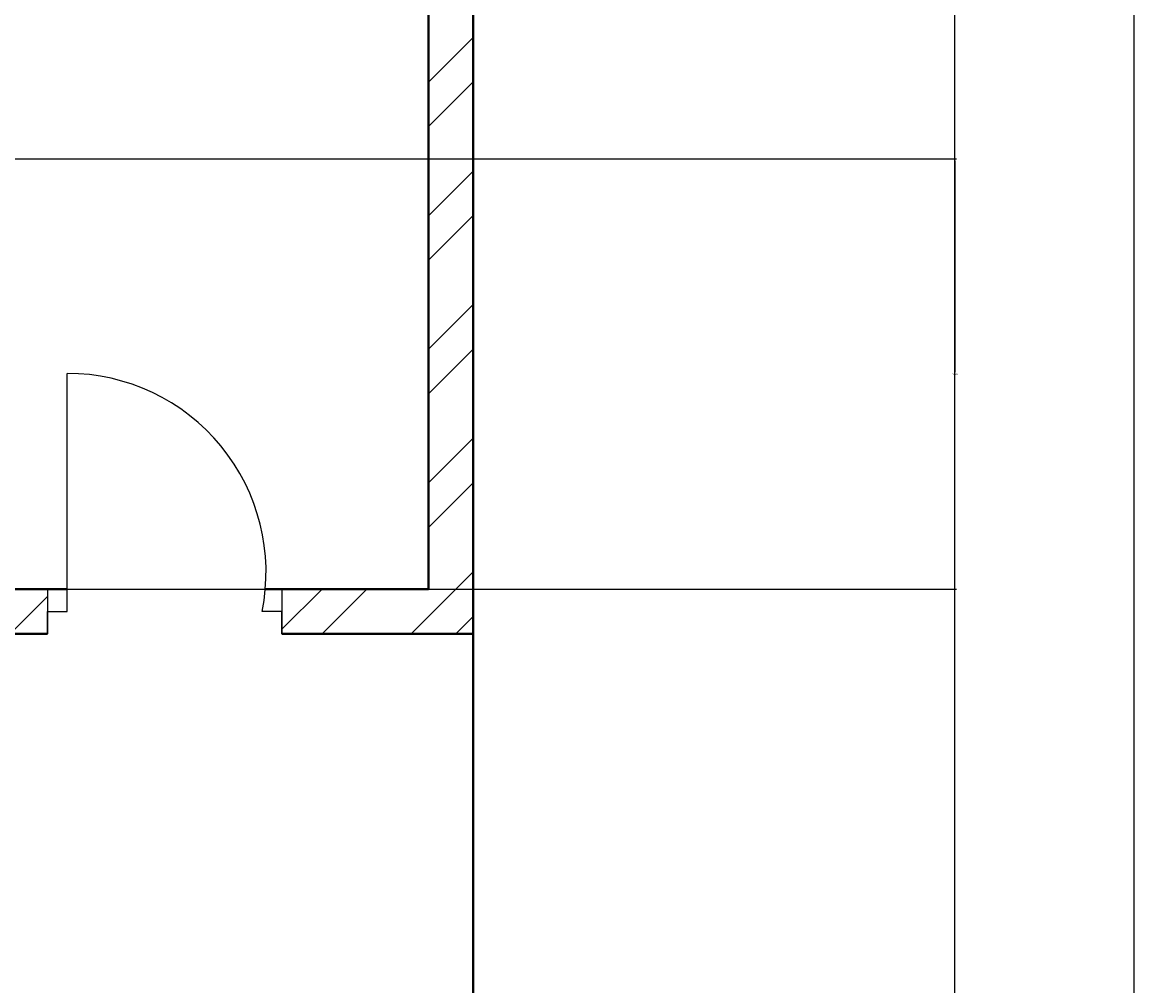
# Model space of a CAD drawing. Units: inches. Extents: x 1601 to 2297, y 1496 to 2631.
# Tile 30 of 57: x 2185 to 2297, y 1946 to 2043. Entities that reach past the tile are written whole.
import ezdxf

# ---------------------------------------------------------------- set-up
doc = ezdxf.new("R2010")
doc.units = ezdxf.units.IN
for name, color, linetype, lineweight in [('A-ANNO-DIMS', 2, 'Continuous', 18), ('A-ANNO-TTLB', 7, 'Continuous', 25), ('A-DOOR', 21, 'Continuous', 25), ('A-WALL', 7, 'Continuous', 40), ('A-WALL-PATT', 215, 'Continuous', 13)]:
    doc.layers.add(name, color=color, linetype=linetype, lineweight=lineweight)
doc.styles.get("Standard").update_dxf_attribs({"font": 'arial.ttf'})
doc.dimstyles.get("Standard").update_dxf_attribs({"dimtxt": 0.18, "dimasz": 0.18, "dimexe": 0.18, "dimexo": 0.0625, "dimgap": 0.09, "dimtad": 0, "dimtih": 1, "dimtoh": 1, "dimdec": 4, "dimzin": 0, "dimdsep": 46, "dimtxsty": 'Standard', "dimcen": 0.09, "dimadec": 0, "dimazin": 0, "dimtfac": 1, "dimtdec": 4, "dimtofl": 0, "dimtmove": 0, "dimatfit": 3, "dimfxl": 1, "dimtolj": 1, "dimtzin": 0, "dimarcsym": 0})

# ---------------------------------------------------------------- blocks, each defined once
blk = doc.blocks.new('*D29')
at = {"layer": 'A-ANNO-DIMS', "color": 0, "lineweight": -2, "transparency": 16777216}
for p, q in [((2230.6, 2532.33), (2279.27, 2532.33)), ((2279.09, 2532.15), (2279.09, 2084.01)), ((2279.09, 1635.51), (2279.09, 2083.64)), ((2230.6, 1635.33), (2279.27, 1635.33))]:
    blk.add_line(p, q, dxfattribs=at)
at = {"layer": 'A-ANNO-DIMS', "color": 0, "transparency": 16777216}
for points in [[(2279.06, 2532.15), (2279.12, 2532.15), (2279.09, 2532.33)], [(2279.06, 1635.51), (2279.12, 1635.51), (2279.09, 1635.33)]]:
    blk.add_solid(points, dxfattribs=at)
at = {"layer": 'Defpoints', "color": 0, "transparency": 16777216}
for p in [(2230.54, 2532.33), (2279.09, 2532.33), (2230.54, 1635.33)]:
    blk.add_point(p, dxfattribs=at)
at = {"layer": 'A-ANNO-DIMS', "color": 0, "transparency": 16777216, "insert": (2279.09, 2083.83), "char_height": 0.18, "attachment_point": 5}
blk.add_mtext('\\A1;897', dxfattribs=at)
blk = doc.blocks.new('*D43')
at = {"layer": 'A-ANNO-DIMS', "color": 0, "lineweight": -2, "transparency": 16777216}
for p, q in [((2182.6, 2029.7), (2279.27, 2029.7)), ((2279.09, 2029.52), (2279.09, 2008.19)), ((2279.09, 1986.51), (2279.09, 2007.83)), ((2178.1, 1986.33), (2279.27, 1986.33))]:
    blk.add_line(p, q, dxfattribs=at)
at = {"layer": 'A-ANNO-DIMS', "color": 0, "transparency": 16777216}
for points in [[(2279.06, 2029.52), (2279.12, 2029.52), (2279.09, 2029.7)], [(2279.06, 1986.51), (2279.12, 1986.51), (2279.09, 1986.33)]]:
    blk.add_solid(points, dxfattribs=at)
at = {"layer": 'Defpoints', "color": 0, "transparency": 16777216}
for p in [(2182.54, 2029.7), (2178.04, 1986.33), (2279.09, 1986.33)]:
    blk.add_point(p, dxfattribs=at)
at = {"layer": 'A-ANNO-DIMS', "color": 0, "transparency": 16777216, "insert": (2279.09, 2008.01), "char_height": 0.18, "attachment_point": 5}
blk.add_mtext('\\A1;43.37', dxfattribs=at)

msp = doc.modelspace()

# ---------------------------------------------------------------- hatches: boundary and pattern name
at = {"layer": 'A-WALL-PATT'}
h = msp.add_hatch(dxfattribs=at)
h.set_pattern_fill('ANSI32', color=256)
h.paths.add_polyline_path([(2230.5373, 1861.8254), (2182.5373, 1861.8254), (2182.5373, 1885.3637), (2178.0373, 1885.3637), (2178.0373, 1861.8254), (2166.0373, 1861.8254), (2134.5373, 1861.8254), (2130.0373, 1861.8254), (2130.0373, 1841.4682), (2126.8833, 1841.4682), (2126.8833, 1836.9682), (2130.0373, 1836.9682), (2130.0373, 1822.7302), (2134.5373, 1822.7302), (2134.5373, 1857.3254), (2166.0373, 1857.3254), (2226.0373, 1857.3254), (2226.0373, 1846.1155), (2230.5373, 1846.1155)])
h.paths.add_polyline_path([(2226.0373, 1797.3254), (2134.5373, 1797.3254), (2134.5373, 1800.6636), (2132.2873, 1800.6636), (2130.0373, 1800.6636), (2130.0373, 1797.3254), (2130.0373, 1792.8254), (2167.7264, 1792.8254), (2226.0373, 1792.8254)])
h.paths.add_polyline_path([(2230.5373, 1822.1155), (2226.0373, 1822.1155), (2226.0373, 1760.8563), (2230.5373, 1760.8563)])
h.paths.add_polyline_path([(2230.5373, 1700.8563), (2226.0373, 1700.8563), (2226.0373, 1644.3254), (2140.2517, 1644.3254), (2140.2517, 1635.3254), (2230.5373, 1635.3254)])
h.paths.add_polyline_path([(2080.2517, 1639.8254), (2080.2517, 1644.3254), (2035.5373, 1644.3254), (2035.5373, 1792.8254), (2094.0373, 1792.8254), (2094.0373, 1797.3254), (2094.0373, 1836.9682), (2097.1057, 1836.9682), (2097.1057, 1839.2182), (2097.1057, 1841.4682), (2094.0373, 1841.4682), (2094.0373, 1862.2276), (2089.5373, 1862.2276), (2089.5373, 1797.3254), (2035.5373, 1797.3254), (2035.5373, 1857.3254), (2035.5373, 1885.0916), (2031.0373, 1885.0916), (2031.0373, 1710.3254), (2012.329, 1710.3254), (2012.329, 1701.3254), (2031.0373, 1701.3254), (2031.0373, 1644.3254), (2031.0373, 1635.3254), (2080.2517, 1635.3254)])
h.paths.add_polyline_path([(1836.0373, 1653.2033), (1842.6171, 1653.2033), (1842.6171, 1657.7033), (1842.6171, 1662.2033), (1831.5373, 1662.2033), (1831.5373, 1764.2033), (1835.3881, 1764.2033), (1835.3881, 1766.4533), (1835.3881, 1768.7033), (1831.5373, 1768.7033), (1827.0373, 1768.7033), (1827.0373, 1662.2033), (1827.0373, 1635.3254), (1836.0373, 1635.3254)])
h.paths.add_polyline_path([(1893.0373, 1701.3254), (1907.193, 1701.3254), (1907.193, 1705.8254), (1907.193, 1710.3254), (1893.0373, 1710.3254), (1893.0373, 1819.8254), (1882.6444, 1819.8254), (1882.6444, 1817.5754), (1882.6444, 1815.3254), (1888.5373, 1815.3254), (1888.5373, 1662.2033), (1884.0373, 1662.2033), (1866.6171, 1662.2033), (1866.6171, 1653.2033), (1882.391, 1653.2033), (1884.0373, 1653.2033), (1884.0373, 1635.3254), (1893.0373, 1635.3254)])
h.paths.add_polyline_path([(1739.3335, 1639.8254), (1739.3335, 1644.3254), (1695.0373, 1644.3254), (1695.0373, 1702.0135), (1690.5373, 1702.0135), (1686.0373, 1702.0135), (1686.0373, 1635.3254), (1739.3335, 1635.3254)])
h.paths.add_polyline_path([(1827.0373, 1644.3254), (1799.3335, 1644.3254), (1799.3335, 1635.3254), (1827.0373, 1635.3254)])
h.paths.add_polyline_path([(1695.0373, 1815.3254), (1849.2759, 1815.3254), (1849.2759, 1819.8254), (1807.5373, 1819.8254), (1807.5373, 1879.8254), (1851.1533, 1879.8254), (1851.1533, 1882.0754), (1851.1533, 1884.3254), (1799.3405, 1884.3254), (1799.3405, 1882.0754), (1799.3405, 1879.8254), (1803.0373, 1879.8254), (1803.0373, 1819.8254), (1695.0373, 1819.8254), (1695.0373, 1835.0458), (1690.5373, 1835.0458), (1686.0373, 1835.0458), (1686.0373, 1766.1753), (1695.0373, 1766.1753)])
h.paths.add_polyline_path([(1775.8157, 1884.3254), (1695.0373, 1884.3254), (1695.0373, 1912.9526), (1690.5373, 1912.9526), (1686.0373, 1912.9526), (1686.0373, 1859.0458), (1695.0373, 1859.0458), (1695.0373, 1879.8254), (1775.8157, 1879.8254)])
h.paths.add_polyline_path([(1893.0373, 2031.3254), (1731.5687, 2031.3254), (1731.5687, 2057.4352), (1722.5687, 2057.4352), (1722.5687, 2031.3254), (1686.0373, 2031.3254), (1686.0373, 1972.9526), (1695.0373, 1972.9526), (1695.0373, 2022.3254), (1888.5373, 2022.3254), (1888.5373, 1884.3254), (1883.4996, 1884.3254), (1883.4996, 1879.8254), (1893.0373, 1879.8254), (1893.0373, 1974.3254), (1976.6199, 1974.3254), (1976.6199, 1978.8254), (1968.0373, 1978.8254), (1968.0373, 1983.3254), (1968.0373, 2008.4756), (1963.5373, 2008.4756), (1959.0373, 2008.4756), (1959.0373, 1983.3254), (1893.0373, 1983.3254)])
h.paths.add_polyline_path([(2230.5373, 2140.4745), (2226.0373, 2140.4745), (2226.0373, 2094.3254), (2040.0373, 2094.3254), (2040.0373, 2085.3254), (2178.0373, 2085.3254), (2178.0373, 2065.6965), (2182.5373, 2065.6965), (2182.5373, 2085.3254), (2226.0373, 2085.3254), (2226.0373, 1986.3254), (2211.2679, 1986.3254), (2211.2679, 1981.8254), (2230.5373, 1981.8254)])
h.paths.add_polyline_path([(2187.6292, 1986.3254), (2182.5373, 1986.3254), (2182.5373, 2029.6965), (2178.0373, 2029.6965), (2178.0373, 1986.3254), (2099.05, 1986.3254), (2099.05, 1981.8254), (2178.0373, 1981.8254), (2178.0373, 1969.3637), (2182.5373, 1969.3637), (2182.5373, 1981.8254), (2187.6292, 1981.8254), (2187.6292, 1984.0754)])
h.paths.add_polyline_path([(1807.1169, 1573.5395), (2055.0405, 1573.5395), (2055.0405, 1610.6322), (1807.1169, 1610.6322)], flags=9)
h.paths.add_polyline_path([(1841.1631, 1712.7967), (1870.3957, 1712.7967), (1870.3957, 1731.454), (1841.1631, 1731.454)], flags=9)
h.paths.add_polyline_path([(2144.3862, 1772.185), (2191.0233, 1772.185), (2191.0233, 1790.8423), (2144.3862, 1790.8423)], flags=9)
h.paths.add_polyline_path([(2143.0128, 1827.3312), (2177.9958, 1827.3312), (2177.9958, 1845.9886), (2143.0128, 1845.9886)], flags=25)
h.paths.add_polyline_path([(2041.2439, 1833.5691), (2070.8516, 1833.5691), (2070.8516, 1852.2264), (2041.2439, 1852.2264)], flags=25)
h.paths.add_polyline_path([(2097.2791, 1947.0598), (2134.2061, 1947.0598), (2134.2061, 1965.7171), (2097.2791, 1965.7171)], flags=9)
h.paths.add_polyline_path([(2214.995, 1904.3124), (2214.995, 1942.2899), (2196.3376, 1942.2899), (2196.3376, 1904.3124)], flags=9)
h.paths.add_polyline_path([(2186.6284, 2043.8031), (2219.7935, 2043.8031), (2219.7935, 2062.4605), (2186.6284, 2062.4605)], flags=25)
h.paths.add_polyline_path([(2064.0877, 2031.616), (2097.4949, 2031.616), (2097.4949, 2050.2734), (2064.0877, 2050.2734)], flags=25)
h.paths.add_polyline_path([(1973.1349, 1986.0688), (2008.4009, 1986.0688), (2008.4009, 2004.7261), (1973.1349, 2004.7261)], flags=9)
h.paths.add_polyline_path([(1976.3676, 2106.9635), (2005.7469, 2106.9635), (2005.7469, 2125.6209), (1976.3676, 2125.6209)], flags=9)
h.paths.add_polyline_path([(1991.7852, 2180.4863), (2027.0513, 2180.4863), (2027.0513, 2199.1437), (1991.7852, 2199.1437)], flags=9)
h.paths.add_polyline_path([(2106.1801, 2187.9359), (2152.2101, 2187.9359), (2152.2101, 2206.5932), (2106.1801, 2206.5932)], flags=9)
h.paths.add_polyline_path([(2148.6686, 2262.2542), (2182.318, 2262.2542), (2182.318, 2280.9115), (2148.6686, 2280.9115)], flags=9)
h.paths.add_polyline_path([(2041.6327, 2252.8147), (2071.2405, 2252.8147), (2071.2405, 2271.4721), (2041.6327, 2271.4721)], flags=9)
h.paths.add_polyline_path([(2063.9734, 2375.4265), (2100.9004, 2375.4265), (2100.9004, 2394.0839), (2063.9734, 2394.0839)], flags=9)
h.paths.add_polyline_path([(2216.4955, 2330.9748), (2216.4955, 2370.2654), (2197.8381, 2370.2654), (2197.8381, 2330.9748)], flags=9)
h.paths.add_polyline_path([(2179.1416, 2485.8687), (2212.3067, 2485.8687), (2212.3067, 2504.5261), (2179.1416, 2504.5261)], flags=9)
h.paths.add_polyline_path([(2078.7442, 2471.1516), (2112.1514, 2471.1516), (2112.1514, 2489.809), (2078.7442, 2489.809)], flags=9)
h.paths.add_polyline_path([(1915.9631, 2329.4668), (1952.8902, 2329.4668), (1952.8902, 2348.1241), (1915.9631, 2348.1241)], flags=9)
h.paths.add_polyline_path([(1904.3189, 2499.6709), (1940.4512, 2499.6709), (1940.4512, 2518.3282), (1904.3189, 2518.3282)], flags=9)
h.paths.add_polyline_path([(1892.3665, 2100.4595), (1925.6374, 2100.4595), (1925.6374, 2119.1169), (1892.3665, 2119.1169)], flags=9)
h.paths.add_polyline_path([(1909.2984, 1805.9631), (1946.2254, 1805.9631), (1946.2254, 1824.6205), (1909.2984, 1824.6205)], flags=9)
h.paths.add_polyline_path([(1934.6056, 1658.616), (1970.738, 1658.616), (1970.738, 1677.2733), (1934.6056, 1677.2733)], flags=9)
h.paths.add_polyline_path([(1711.2052, 1789.8902), (1750.0456, 1789.8902), (1750.0456, 1808.5476), (1711.2052, 1808.5476)], flags=25)
h.paths.add_polyline_path([(1742.7874, 1854.6743), (1771.9449, 1854.6743), (1771.9449, 1873.3317), (1742.7874, 1873.3317)], flags=25)
h.paths.add_polyline_path([(1807.3592, 1997.7912), (1850.1116, 1997.7912), (1850.1116, 2016.4486), (1807.3592, 2016.4486)], flags=25)
h.paths.add_polyline_path([(1717.4579, 2237.7844), (1760.2103, 2237.7844), (1760.2103, 2256.4417), (1717.4579, 2256.4417)], flags=9)
h.paths.add_polyline_path([(1780.9285, 2324.0623), (1810.086, 2324.0623), (1810.086, 2342.7197), (1780.9285, 2342.7197)], flags=9)
h.paths.add_polyline_path([(1837.696, 2449.2024), (1866.9286, 2449.2024), (1866.9286, 2467.8598), (1837.696, 2467.8598)], flags=9)
h.paths.add_polyline_path([(1712.7752, 2484.9404), (1751.6156, 2484.9404), (1751.6156, 2503.5977), (1712.7752, 2503.5977)], flags=9)

# ---------------------------------------------------------------- linework, layer by layer
at = {"layer": 'A-ANNO-TTLB'}
msp.add_lwpolyline([(1600.5933, 2631.1477), (2297.129, 2631.1477), (2297.129, 1496.1026), (1600.5933, 1496.1026)], close=True, dxfattribs=at)
at = {"layer": 'A-DOOR'}
for p, q in [((2189.6292, 1984.0754), (2189.6292, 2008.0754)), ((2187.6292, 1986.3254), (2187.6292, 1981.8254)), ((2211.2679, 1986.3254), (2211.2679, 1981.8254)), ((2187.6292, 1981.8254), (2187.6292, 1984.0754)), ((2187.6292, 1984.0754), (2189.6292, 1984.0754)), ((2211.2679, 1984.0754), (2209.2679, 1984.0754)), ((2211.2679, 1981.8254), (2211.2679, 1984.0754))]:
    msp.add_line(p, q, dxfattribs=at)
msp.add_arc((2189.6292, 1988.0404), 20.035, 348.585516, 90, dxfattribs=at)
at = {"layer": 'A-WALL'}
for p, q in [((2230.5373, 2140.4745), (2230.5373, 1846.1155)), ((2226.0373, 2085.3254), (2226.0373, 1986.3254)), ((2182.5373, 1986.3254), (2189.6292, 1986.3254)), ((2209.5906, 1986.3254), (2226.0373, 1986.3254)), ((2182.5373, 1981.8254), (2187.6292, 1981.8254)), ((2211.2679, 1981.8254), (2230.5373, 1981.8254))]:
    msp.add_line(p, q, dxfattribs=at)

# ---------------------------------------------------------------- dimensions: what is measured, and where the dimension line sits
at = {"layer": 'A-ANNO-DIMS'}
for base, p1, p2, override, picture, middle in [((2279.0873, 2532.3254), (2230.5373, 1635.3254), (2230.5373, 2532.3254), {"dimdec": 0, "dimlfac": 1, "dimrnd": 0, "dimzin": 0, "dimdsep": 46, "dimlunit": 2}, '*D29', (2279.0873, 2083.8254)), ((2279.0873, 1986.3254), (2182.5373, 2029.6965), (2178.0373, 1986.3254), {"dimdec": 2, "dimlfac": 1, "dimrnd": 0, "dimzin": 0, "dimdsep": 46, "dimlunit": 2}, '*D43', (2279.0873, 2008.011))]:
    dim = msp.add_linear_dim(base=base, p1=p1, p2=p2, angle=90, dimstyle='Standard', override=override, dxfattribs=at)
    dim.commit()
    dim.dimension.update_dxf_attribs({"geometry": picture, "text_midpoint": middle})

doc.saveas('drawing.dxf')
